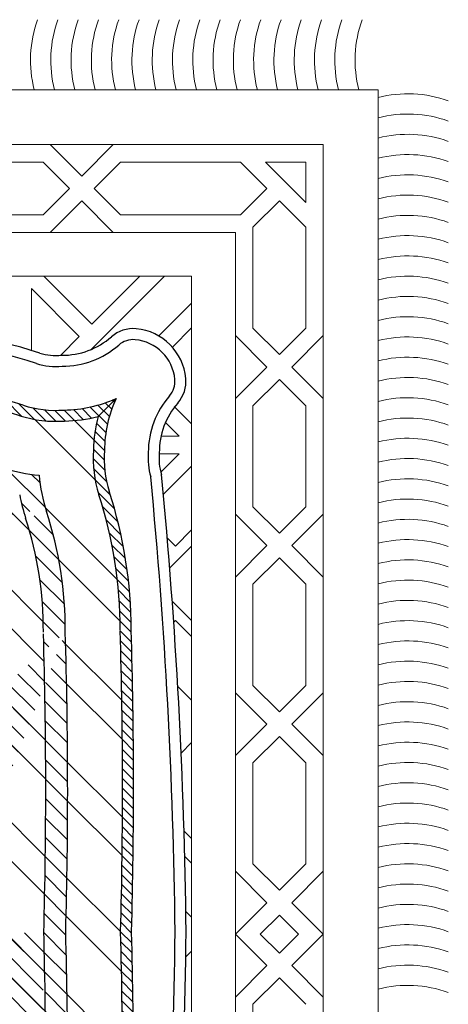
# Model space of a CAD drawing. Units: inches. Extents: x 3592 to 4861, y 1650 to 2243.
# Tile 8 of 30: x 4207 to 4219, y 1932 to 1959. Entities that reach past the tile are written whole.
import ezdxf

# ---------------------------------------------------------------- set-up
doc = ezdxf.new("R2010")
doc.units = ezdxf.units.IN
doc.layers.add('A-FURN', color=9, linetype='Continuous', lineweight=13)
doc.layers.add('RA-AP-01$0$INT', color=35, linetype='Continuous', lineweight=5)
for name, color, linetype in [('RA-AP-01$0$FURN', 3, 'Continuous'), ('RA-AP-01$0$WOOD', 64, 'Continuous'), ('RA-AP-02$0$FLPT', 30, 'Continuous')]:
    doc.layers.add(name, color=color, linetype=linetype)

# ---------------------------------------------------------------- blocks, each defined once
blk = doc.blocks.new('A$C67D63ADA')
at = {"layer": 'RA-AP-01$0$INT'}
for p, q in [((4.360068427138701, -6.272102561815665), (4.331382135641587, -6.243416270309323)), ((4.388754718643982, -6.243416270319609), (4.360068427138701, -6.272102561815665)), ((4.494210562764795, -6.243416270339973), (4.52289685426085, -6.272102561845255)), ((4.551583145766129, -6.243416270324172), (4.522896854260848, -6.272102561820228)), ((4.657038989890581, -6.243416270339336), (4.685725281386635, -6.272102561844619)), ((4.714411572875414, -6.243416270339336), (4.685725281379359, -6.272102561844619)), ((4.819867416996229, -6.243416270324516), (4.848553708501509, -6.272102561820572)), ((4.848553708501509, -6.272102561820572), (4.877239999998625, -6.243416270314227)), ((4.905926291512142, -6.272102561820572), (4.877240000015027, -6.243416270314227)), ((4.934612583017423, -6.243416270324516), (4.905926291512142, -6.272102561820572)), ((4.173240000009217, -6.296102561814969), (4.209926291520478, -6.259416270315509)), ((4.209926291520478, -6.259416270315509), (4.173240000009216, -6.259416270315509)), ((4.173240000009217, -6.296102561814969), (4.173240000009216, -6.259416270315509)), ((4.232553708503005, -6.259416270315509), (4.208553708513718, -6.283416270312518)), ((4.324754718648297, -6.259416270315509), (4.232553708503005, -6.259416270315509)), ((4.348754718637899, -6.283416270312828), (4.324754718648297, -6.259416270315509)), ((4.395382135631553, -6.2594162703285), (4.371382135635868, -6.283416270316472)), ((4.48758314576926, -6.259416270343913), (4.395382135631553, -6.2594162703285)), ((4.48758314576926, -6.259416270343913), (4.511583145760048, -6.283416270342422)), ((4.558210562765816, -6.259416270320948), (4.534210562758016, -6.283416270321034)), ((4.650411572888129, -6.259416270336362), (4.558210562765816, -6.259416270320948)), ((4.650411572888129, -6.259416270336362), (4.674411572885833, -6.283416270341786)), ((4.721038989873787, -6.25941627034044), (4.697038989880161, -6.283416270341786)), ((4.721038989873787, -6.25941627034044), (4.813239999999876, -6.259416270325027)), ((4.813240000000789, -6.259416270325538), (4.837240000004343, -6.283416270321379)), ((4.859867417002312, -6.283416270317736), (4.877240000001861, -6.2660436873126)), ((4.89461258301134, -6.283416270317736), (4.877240000011791, -6.2660436873126)), ((4.941240000012863, -6.259416270325538), (4.917240000009309, -6.283416270321379)), ((4.232553708510282, -6.307416270316805), (4.208553708513718, -6.283416270312518)), ((4.348754718637899, -6.283416270312828), (4.324754718627222, -6.307416270315791)), ((4.395382135640173, -6.307416270328503), (4.371382135635868, -6.283416270316472)), ((4.487583145750843, -6.307416270343915), (4.511583145760048, -6.283416270342422)), ((4.558210562750208, -6.307416270320947), (4.534210562758016, -6.283416270321034)), ((4.650411572883545, -6.307416270336361), (4.674411572885833, -6.283416270341786)), ((4.721038989886534, -6.307416270340442), (4.697038989880161, -6.283416270341786)), ((4.813240000007903, -6.30741627032554), (4.837240000004343, -6.283416270321379)), ((4.859867417002312, -6.283416270317736), (4.877240000006826, -6.300788853316665)), ((4.89461258301134, -6.283416270317736), (4.877240000006826, -6.300788853316665)), ((4.941240000005749, -6.30741627032554), (4.917240000009309, -6.283416270321379)), ((4.173240000009217, -6.318729978809296), (4.19724000000369, -6.294729978822545)), ((4.221240000009218, -6.318729978820355), (4.19724000000369, -6.294729978822545)), ((4.360068427135066, -6.294729978813635), (4.331382135628725, -6.323416270310751)), ((4.388754718631812, -6.323416270319609), (4.360068427135066, -6.294729978813635)), ((4.49421056275124, -6.323416270339973), (4.522896854257212, -6.294729978843224)), ((4.551583145753959, -6.323416270324171), (4.522896854257213, -6.294729978818199)), ((4.657038989877026, -6.323416270339336), (4.685725281382997, -6.294729978842587)), ((4.714411572888969, -6.323416270339336), (4.685725281382997, -6.294729978842587)), ((4.819867417008399, -6.323416270324515), (4.848553708505145, -6.294729978818542)), ((4.848553708505147, -6.29472997881854), (4.877240000011487, -6.323416270315655)), ((4.905926291508504, -6.29472997881854), (4.877240000002164, -6.323416270315655)), ((4.934612583005253, -6.323416270324515), (4.905926291508508, -6.294729978818542)), ((4.232553708510282, -6.307416270316805), (4.324754718627222, -6.307416270315791)), ((4.487583145750843, -6.307416270343915), (4.395382135640173, -6.307416270328503)), ((4.650411572883545, -6.307416270336361), (4.558210562750208, -6.307416270320947)), ((4.721038989886534, -6.307416270340442), (4.813240000007903, -6.307416270325028)), ((5.033441010127117, -6.307416270340442), (4.941240000005749, -6.307416270325028)), ((4.173240000009216, -6.428102561824165), (4.173240000009217, -6.318729978809296)), ((4.221240000009218, -6.428102561821944), (4.221240000009218, -6.318729978820355)), ((4.237240000008252, -6.353816270320467), (4.237240000008252, -6.933016270323148)), ((4.237240000008253, -6.353816270322416), (4.237240000008253, -6.933016270318608)), ((4.277240000006364, -6.923416270324413), (4.277240000021174, -6.363416270332882)), ((4.877240000006826, -6.363416270330311), (4.277240000021174, -6.363416270332882)), ((4.331724248037607, -6.393331975860947), (4.301808542509442, -6.363416270332777)), ((4.324435959507737, -6.36341627033268), (4.341921384137314, -6.380901694962252)), ((4.411867417009952, -6.363416270332308), (4.396098836564792, -6.379184850777471)), ((4.45049483400792, -6.363416270332143), (4.476136761714619, -6.389058198038839)), ((4.508671457515881, -6.363416270331893), (4.45049483400792, -6.363416270332143)), ((4.508671457515881, -6.363416270331891), (4.523298874513887, -6.378043687329895)), ((4.591181125507156, -6.363416270331923), (4.523298874513629, -6.363416270331545)), ((4.543172726528447, -6.383290122346805), (4.523298874513629, -6.363416270331545)), ((4.573619639006339, -6.380977756832742), (4.591181125507156, -6.363416270331923)), ((4.605808542505038, -6.363416270331884), (4.591181125507032, -6.378043687329889)), ((4.591181125507033, -6.378043687329889), (4.605808542505001, -6.363416270331923)), ((4.605808542505038, -6.363416270331886), (4.663985166013, -6.363416270332124)), ((4.663985166013, -6.363416270332124), (4.65146504581717, -6.375936390527956)), ((4.702612583010965, -6.36341627033228), (4.790044040513182, -6.363416270332642)), ((4.702612583010966, -6.363416270332284), (4.712072573448597, -6.372876260769913)), ((4.790044040513182, -6.363416270332642), (4.783212045294504, -6.370248265551321)), ((4.806473209246069, -6.369614518597721), (4.812671457513201, -6.363416270330588)), ((4.856598418256279, -6.368626394577383), (4.861808542503284, -6.363416270330378)), ((4.877240000006826, -6.363416270330311), (5.477239999992479, -6.363416270332882)), ((4.897949975524354, -6.368694788344366), (4.892671457510368, -6.363416270330378)), ((4.423181125509032, -6.374729978831202), (4.410714462749727, -6.387196641590509)), ((4.423181125509103, -6.391217225305457), (4.423181125509032, -6.374729978831202)), ((4.439181125509032, -6.374729978831223), (4.455879744643261, -6.39142859796545)), ((4.43918112550911, -6.392862294450365), (4.439181125509032, -6.374729978831223)), ((4.51581063184268, -6.385531930001103), (4.523298874513885, -6.378043687329895)), ((4.592759677987533, -6.379622239810387), (4.591181125507033, -6.378043687329889)), ((4.344016470827723, -6.454761283640936), (4.277240000020523, -6.387984812833736)), ((4.277240000019926, -6.410612229819946), (4.320955728769878, -6.454327958571846)), ((4.173240000009216, -6.428102561824165), (4.197240000007798, -6.452102561823052)), ((4.221240000009218, -6.428102561821944), (4.197240000007798, -6.452102561823052)), ((4.157240000008254, -6.434729978821112), (4.185926291507684, -6.463416270320908)), ((4.237240000008253, -6.434729978820932), (4.20855370850791, -6.46341627032091)), ((4.277240000017616, -6.498043687322161), (4.320955728769878, -6.454327958571846)), ((4.157240000008254, -6.492102561820703), (4.185926291507684, -6.463416270320908)), ((4.237240000008253, -6.492102561820884), (4.20855370850791, -6.46341627032091)), ((4.28855370851626, -6.509357395821494), (4.332269437268611, -6.465641667071082)), ((4.332269437268613, -6.465641667071083), (4.349438136078297, -6.482810365881532)), ((4.173240000008253, -6.498729978818613), (4.197240000007798, -6.474729978818764)), ((4.221240000008254, -6.498729978818907), (4.197240000007798, -6.474729978818764)), ((4.173240000008255, -6.608102561821608), (4.173240000008253, -6.498729978818613)), ((4.221240000008257, -6.608102561821311), (4.221240000008254, -6.498729978818907)), ((4.344903410716357, -6.509357395822983), (4.28855370851626, -6.509357395821494))]:
    blk.add_line(p, q, dxfattribs=at)
for points in [[(5.647240000006826, -6.243416270325369), (5.647240000006826, -7.09341627032537), (4.107240000006826, -7.093416270325372), (4.107240000006826, -6.19341627032537), (4.877240000006826, -6.19341627032537)], [(4.877240000006826, -6.19341627032537), (5.647240000006826, -6.19341627032537), (5.647240000006826, -7.09341627032537), (4.877240000006826, -7.09341627032537)], [(5.597240000006826, -6.243416270325369), (5.597240000006826, -7.04341627032537), (4.157240000006826, -7.043416270325372), (4.157240000006826, -6.243416270325369)], [(4.877240000006826, -6.243416270325369), (4.157240000006826, -6.243416270325369)], [(4.877240000006826, -6.243416270325369), (5.597240000006826, -6.243416270325369)], [(4.877240000006826, -6.32341627032537), (4.237240000006825, -6.32341627032537), (4.237240000006825, -6.963416270325371), (4.877240000006826, -6.963416270325371)], [(4.877240000006826, -6.32341627032537), (5.517240000006826, -6.32341627032537), (5.517240000006826, -6.963416270325371), (4.877240000006826, -6.963416270325371)]]:
    blk.add_lwpolyline(points, dxfattribs=at)
for centre, start, end in [((4.220001958960506, -6.166456270323309), 160.2038431294313, 194.3025426369059), ((4.238481958959505, -6.166456270325492), 160.2038431294313, 194.302542635723), ((4.256961958958505, -6.166456270325492), 160.2038431294313, 194.302542635723), ((4.275441958962233, -6.166456270324219), 160.2038431294313, 194.3025426364132), ((4.293921958961232, -6.166456270326402), 160.2038431294313, 194.3025426352303), ((4.312401958960231, -6.166456270326402), 160.2038431294313, 194.3025426352303), ((4.33088195896396, -6.166456270325128), 160.2038431294313, 194.3025426359204), ((4.349361958962959, -6.166456270326038), 160.2038431294313, 194.3025426354275), ((4.367841958959411, -6.166456270326038), 160.2038431294313, 194.3025426354275), ((4.386321958963322, -6.166456270324765), 160.2038431294313, 194.3025426361172), ((4.404801958962321, -6.166456270326947), 160.2038431294313, 194.3025426349348), ((4.42328195896132, -6.166456270326947), 160.2038431294313, 194.3025426349348), ((4.441761958965049, -6.166456270325674), 160.2038431294313, 194.3025426356244), ((4.460241958964048, -6.166456270326584), 160.2038431294313, 194.3025426351316), ((4.4787219589605, -6.166456270326584), 160.2038431294313, 194.3025426351316), ((4.497201958964411, -6.16645627032531), 160.2038431294313, 194.3025426358216), ((4.515681958963228, -6.166456270323855), 160.2038431294313, 194.3025426366099), ((4.534161958959862, -6.16645627032622), 160.2038431294313, 194.3025426353289), ((4.552641958963591, -6.166456270326038), 160.2038431294313, 194.3025426354275), ((4.571121958962589, -6.166456270324765), 160.2038431294313, 194.3025426361172), ((4.589601958963954, -6.166456270323491), 160.2038431294313, 194.3025426368072), ((4.608081958962952, -6.166456270325674), 160.2038431294313, 194.3025426356244), ((4.626561958963465, -6.166456270323128), 160.2038431294313, 194.3025426370041), ((4.626561958964317, -6.166456270325492), 160.2038431294313, 194.302542635723), ((4.645041958962464, -6.16645627032531), 160.2038431294313, 194.3025426358216), ((4.663521958961464, -6.16645627032531), 160.2038431294313, 194.3025426358216), ((4.682001958965192, -6.166456270324037), 160.2038431294313, 194.3025426365113), ((4.700481958964191, -6.166456270324947), 160.2038431294313, 194.3025426360186), ((4.718961958960644, -6.166456270324947), 160.2038431294313, 194.3025426360186), ((4.737441958964554, -6.166456270323673), 160.2038431294313, 194.3025426367086), ((4.755921958963371, -6.166456270322218), 160.2038431294313, 194.3025426374968), ((4.774401958960006, -6.166456270324583), 160.2038431294313, 194.3025426362158), ((4.792881958963734, -6.166456270324401), 160.2038431294313, 194.3025426363144), ((4.811361958962733, -6.166456270323128), 160.2038431294313, 194.3025426370041), ((4.829841958964097, -6.166456270321854), 160.2038431294313, 194.3025426376941), ((4.848321958963096, -6.166456270324037), 160.2038431294313, 194.3025426365113), ((4.86680195896446, -6.166456270323855), 160.2038431294313, 194.3025426366099), ((4.885281958960913, -6.16645627032149), 160.2038431294313, 194.3025426378914), ((4.903761958964823, -6.166456270321309), 160.2038431294313, 194.3025426379896), ((4.92224195896364, -6.166456270323673), 160.2038431294313, 194.3025426367086), ((4.940721958962639, -6.1664562703224), 160.2038431294313, 194.3025426373987), ((4.959201958964003, -6.166456270320945), 160.2038431294313, 194.3025426381869), ((4.977681958963002, -6.166456270320945), 160.2038431294313, 194.3025426381869), ((4.996161958962002, -6.166456270323128), 160.2038431294313, 194.3025426370041), ((5.014641958961001, -6.166456270323128), 160.2038431294313, 194.3025426370041), ((5.033121958964729, -6.166456270321854), 160.2038431294313, 194.3025426376941), ((4.080280000008716, -6.105294311367939), 250.2038431288995, 284.3025426347654), ((4.080280000011353, -6.123774311370394), 250.2038431288995, 284.3025426333367), ((4.080280000008989, -6.142254311367028), 250.2038431288995, 284.3025426346176), ((4.080280000006625, -6.160734311363481), 250.2038431288995, 284.3025426358987), ((4.080280000009262, -6.179214311365936), 250.2038431288995, 284.3025426344699), ((4.080280000006897, -6.19769431136257), 250.2038431288995, 284.302542635751), ((4.080280000004532, -6.216174311359023), 250.2038431288995, 284.3025426370325), ((4.080280000007079, -6.234654311360387), 250.2038431288995, 284.3025426356524), ((4.08028000000726, -6.253134311360659), 250.2038431288995, 284.3025426355542), ((4.08028000000726, -6.271614311362022), 250.2038431288995, 284.3025426355542), ((4.080280000005078, -6.290094311364478), 250.2038431288995, 284.3025426367365), ((4.080280000007534, -6.30857431136475), 250.2038431288995, 284.302542635406), ((4.080280000007625, -6.327054311362476), 250.2038431288995, 284.3025426353568), ((4.080280000005441, -6.345534311362567), 250.2038431288995, 284.3025426365397), ((4.080280000005533, -6.364014311362839), 250.2038431288995, 284.3025426364901), ((4.080280000005624, -6.382494311361838), 250.2038431288995, 284.302542636441), ((4.08028000000817, -6.400974311363202), 250.2038431288995, 284.3025426350613)]:
    blk.add_arc(centre, 0.1091312342836184, start, end, dxfattribs=at)
blk = doc.blocks.new('A$C09A87C41')
at = {"layer": 'RA-AP-01$0$WOOD'}
h = blk.add_hatch(dxfattribs=at)
h.set_pattern_fill('ANSI31', color=256, scale=0.05, style=0)
h.set_pattern_definition([(45, (0.7182879904584168, -11.54818755465011), (0.0044194173824159, -0.0044194173824159), [])])
edge = h.paths.add_edge_path()
edge.add_ellipse((5.006516613079209, -11.27459283286495), major_axis=(3.435359877543153, 3.435359877543153), ratio=0.9999999999999982, start_angle=403.3022422558093, end_angle=406.5486575131389, ccw=False)
edge.add_ellipse((5.150455045735207, -6.828790194879051), major_axis=(-0.2901946312779826, 0.2901946312779826), ratio=0.9999999999999875, start_angle=297.2093186994243, end_angle=314.9999999999731, ccw=False)
edge.add_ellipse((5.307117976013378, -6.343033378039902), major_axis=(-0.0707106781186454, 0.0707106781186455), ratio=0.9999999999999651, start_angle=116.7779839927149, end_angle=139.0873288843009)
edge.add_ellipse((5.312718414970339, -6.324818905441738), major_axis=(0.0834173982641243, 0.0834173982641243), ratio=0.9999999999999847, start_angle=225.741775187377, end_angle=249.5633269497028)
edge.add_line((5.361758401537698, -6.432112914518591), (5.345299417747169, -6.448571898309089))
edge.add_ellipse((5.312718414970311, -6.32481890544173), major_axis=(-0.0904884660759946, 0.0904884660759945), ratio=0.9999999999999644, start_angle=135.8720682536374, end_angle=149.7498089726665, ccw=False)
edge.add_ellipse((5.307117976013483, -6.343033378039922), major_axis=(-0.0777817459304867, 0.0777817459304867), ratio=0.9999999999999941, start_angle=117.45144083316339, end_angle=138.9346900893823, ccw=False)
edge.add_ellipse((5.150455045735208, -6.82879019487905), major_axis=(0.2831235634661059, 0.2831235634661059), ratio=0.9999999999999859, start_angle=27.03507540014952, end_angle=44.9867285887044)
edge.add_ellipse((5.006516315412802, -11.27459997798134), major_axis=(-3.428298916554014, 3.428298916554014), ratio=0.9999999999999971, start_angle=-46.70235550375367, end_angle=-43.44815559494434)
edge.add_ellipse((4.743915471599394, -11.2745999779814), major_axis=(3.428298916553931, 3.42829891655393), ratio=0.9999999999999994, start_angle=43.44815559494427, end_angle=46.70235550375375)
edge.add_ellipse((4.599976741276995, -6.828790194879051), major_axis=(0.2831235634661173, 0.2831235634661172), ratio=0.9999999999999861, start_angle=45.01327141129749, end_angle=62.96492459984043)
edge.add_ellipse((4.443313810998718, -6.343033378039922), major_axis=(0.0777817459304893, 0.0777817459304893), ratio=0.9999999999999873, start_angle=221.0653099106178, end_angle=242.54855916687399, ccw=False)
edge.add_ellipse((4.437713372041892, -6.32481890544173), major_axis=(0.0904884660759951, 0.0904884660759951), ratio=0.9999999999999603, start_angle=210.2501910273332, end_angle=224.1279317463614, ccw=False)
edge.add_line((4.405132369265034, -6.448571898309089), (4.388673385474508, -6.432112914518594))
edge.add_ellipse((4.43771337204186, -6.324818905441737), major_axis=(0.0834173982641232, 0.0834173982641232), ratio=0.9999999999999797, start_angle=200.4366730503009, end_angle=224.2582248126243)
edge.add_ellipse((4.443313810998827, -6.343033378039902), major_axis=(-0.0707106781186382, 0.0707106781186382), ratio=0.9999999999999952, start_angle=130.9126711156974, end_angle=153.2220160072772)
edge.add_ellipse((4.599976741276995, -6.828790194879051), major_axis=(-0.2901946312779718, 0.2901946312779718), ratio=0.9999999999999895, start_angle=315.0000000000233, end_angle=332.7906813005773, ccw=False)
edge.add_ellipse((4.743915173933024, -11.27459283286497), major_axis=(-3.435359877543123, 3.435359877543123), ratio=0.9999999999999991, start_angle=313.451342486861, end_angle=316.69775774419077, ccw=False)
edge = h.paths.add_edge_path()
edge.add_ellipse((4.299593848995801, -6.48675334004306), major_axis=(-0.0707106781186556, 0.0707106781186556), ratio=0.9999999999999859, start_angle=206.7779839906583, end_angle=229.0873288838364)
edge.add_ellipse((4.281379376397651, -6.481152901086075), major_axis=(-0.0834173982641623, 0.0834173982641623), ratio=0.9999999999999754, start_angle=225.7417751869729, end_angle=249.5633269497573)
edge.add_line((4.388673385474506, -6.432112914518592), (4.405132369265034, -6.448571898309089))
edge.add_ellipse((4.281379376397657, -6.481152901086004), major_axis=(-0.0904884660760182, 0.0904884660760182), ratio=0.9999999999999957, start_angle=225.8720682533453, end_angle=239.7498089726896, ccw=False)
edge.add_ellipse((4.299593848995796, -6.486753340043026), major_axis=(0.0777817459305317, 0.0777817459305317), ratio=0.9999999999999891, start_angle=297.4514408381613, end_angle=318.9346900891407, ccw=False)
edge.add_ellipse((4.785350665835052, -6.643416270320893), major_axis=(0.2831235634661102, 0.2831235634661102), ratio=0.9999999999999978, start_angle=117.0350753988375, end_angle=152.9649246009711)
edge.add_ellipse((4.299593848995777, -6.800079200598784), major_axis=(-0.0777817459305426, 0.0777817459305426), ratio=0.9999999999999973, start_angle=221.0653099111909, end_angle=242.5485591625442, ccw=False)
edge.add_ellipse((4.281379376397679, -6.805679639555494), major_axis=(-0.0904884660760244, 0.0904884660760244), ratio=0.9999999999999076, start_angle=210.2501910270576, end_angle=224.1279317467988, ccw=False)
edge.add_line((4.405132369264926, -6.838260642332959), (4.388673385474263, -6.854719626123697))
edge.add_ellipse((4.281379376397679, -6.80567963955562), major_axis=(0.0834173982641642, 0.0834173982641642), ratio=0.9999999999999609, start_angle=290.4366730499258, end_angle=314.2582248131156)
edge.add_ellipse((4.299593848995804, -6.800079200598786), major_axis=(-0.0707106781186612, 0.0707106781186612), ratio=0.999999999999977, start_angle=220.9126711163551, end_angle=243.222016008517)
edge.add_ellipse((4.785350665835053, -6.643416270320894), major_axis=(0.2901946312779783, 0.2901946312779783), ratio=0.9999999999999984, start_angle=117.2093186999746, end_angle=152.7906813002342, ccw=False)
edge = h.paths.add_edge_path()
edge.add_ellipse((4.743915471599392, -2.012232562660299), major_axis=(3.428298916553894, 3.428298916553894), ratio=0.9999999999999992, start_angle=223.2976444962459, end_angle=226.5518444050561)
edge.add_ellipse((5.006516315412771, -2.012232562660296), major_axis=(3.428298916553752, 3.428298916553752), ratio=0.9999999999999971, start_angle=223.448155594945, end_angle=226.7023555037531)
edge.add_ellipse((5.150455045735209, -6.458042345762599), major_axis=(0.283123563466111, 0.283123563466111), ratio=0.999999999999996, start_angle=225.0132714112834, end_angle=242.9649246011241)
edge.add_ellipse((5.30711797601273, -6.94379916260194), major_axis=(0.0777817459305174, 0.0777817459305174), ratio=0.9999999999999873, start_angle=401.06530991071423, end_angle=422.548559161793, ccw=False)
edge.add_ellipse((5.312718414969516, -6.962013635200094), major_axis=(0.0904884660760023, 0.0904884660760023), ratio=0.9999999999999566, start_angle=390.2501910269164, end_angle=404.12793174642553, ccw=False)
edge.add_line((5.345299417747278, -6.838260642332959), (5.361758401537942, -6.854719626123698))
edge.add_ellipse((5.312718414969516, -6.962013635200098), major_axis=(0.0834173982641439, 0.0834173982641439), ratio=0.9999999999999785, start_angle=20.43667304973462, end_angle=44.25822481258737)
edge.add_ellipse((5.307117976012772, -6.943799162601948), major_axis=(-0.0707106781186618, 0.0707106781186618), ratio=0.999999999999977, start_angle=-49.08732888421749, end_angle=-26.77798399064677)
edge.add_ellipse((5.150455045735209, -6.458042345762597), major_axis=(0.2901946312779783, 0.2901946312779783), ratio=0.9999999999999957, start_angle=225.0000000000273, end_angle=242.7906812999824, ccw=False)
edge.add_ellipse((5.006516613079198, -2.012239707776725), major_axis=(3.43535987754352, 3.43535987754352), ratio=0.999999999999996, start_angle=223.4513424868609, end_angle=226.697757744191, ccw=False)
edge.add_ellipse((4.743915173933023, -2.012239707776712), major_axis=(3.435359877543229, 3.435359877543229), ratio=0.9999999999999998, start_angle=223.3022422558095, end_angle=226.5486575131387, ccw=False)
edge.add_ellipse((4.599976741276995, -6.458042345762597), major_axis=(0.2901946312779746, 0.2901946312779748), ratio=0.9999999999999964, start_angle=207.2093187000184, end_angle=224.9999999999795, ccw=False)
edge.add_ellipse((4.443313810999427, -6.943799162601947), major_axis=(-0.070710678118668, 0.070710678118668), ratio=0.9999999999999838, start_angle=-63.22201600935903, end_angle=-40.9126711157662)
edge.add_ellipse((4.437713372042683, -6.962013635200099), major_axis=(0.0834173982641484, 0.0834173982641484), ratio=0.9999999999999729, start_angle=45.74177518742643, end_angle=69.56332695026246)
edge.add_line((4.388673385474263, -6.854719626123697), (4.405132369264926, -6.838260642332958))
edge.add_ellipse((4.437713372042681, -6.962013635200094), major_axis=(0.0904884660760224, 0.0904884660760225), ratio=0.9999999999999282, start_angle=405.87206825357924, end_angle=419.7498089730807, ccw=False)
edge.add_ellipse((4.443313810999475, -6.94379916260194), major_axis=(-0.0777817459305165, 0.0777817459305165), ratio=0.9999999999999927, start_angle=297.4514408382556, end_angle=318.93469008929503, ccw=False)
edge.add_ellipse((4.599976741276995, -6.458042345762597), major_axis=(0.2831235634661077, 0.2831235634661077), ratio=0.9999999999999937, start_angle=207.0350753988627, end_angle=224.9867285886981)
edge = h.paths.add_edge_path()
edge.add_ellipse((5.450837938016399, -6.800079200598789), major_axis=(-0.0707106781186565, 0.0707106781186565), ratio=0.9999999999999875, start_angle=26.77798399147072, end_angle=49.08732888364846)
edge.add_ellipse((5.469052410614524, -6.80567963955562), major_axis=(0.0834173982641601, 0.0834173982641601), ratio=0.9999999999999984, start_angle=135.7417751868887, end_angle=159.563326950074)
edge.add_line((5.36175840153794, -6.854719626123697), (5.345299417747278, -6.838260642332959))
edge.add_ellipse((5.469052410614523, -6.805679639555488), major_axis=(0.0904884660760307, 0.0904884660760307), ratio=0.9999999999999984, start_angle=135.8720682531977, end_angle=149.7498089729454, ccw=False)
edge.add_ellipse((5.450837938016426, -6.800079200598787), major_axis=(0.0777817459305426, 0.0777817459305427), ratio=0.9999999999999968, start_angle=117.4514408374904, end_angle=138.9346900888003, ccw=False)
edge.add_ellipse((4.965081121177151, -6.643416270320895), major_axis=(-0.2831235634661119, 0.2831235634661119), ratio=0.9999999999999992, start_angle=207.0350753990193, end_angle=242.9649246011595)
edge.add_ellipse((5.450837938016407, -6.486753340043026), major_axis=(0.0777817459305285, 0.0777817459305285), ratio=0.9999999999999747, start_angle=131.0653099108597, end_angle=152.5485591618505, ccw=False)
edge.add_ellipse((5.469052410614547, -6.481152901086004), major_axis=(0.09048846607603, 0.09048846607603), ratio=0.9999999999999619, start_angle=120.25019102731059, end_angle=134.1279317466551, ccw=False)
edge.add_line((5.345299417747169, -6.448571898309089), (5.361758401537697, -6.432112914518592))
edge.add_ellipse((5.469052410614551, -6.481152901086075), major_axis=(-0.0834173982641603, 0.0834173982641603), ratio=0.9999999999999998, start_angle=20.43667305024269, end_angle=44.25822481302925)
edge.add_ellipse((5.450837938016403, -6.486753340043062), major_axis=(-0.0707106781186603, 0.0707106781186603), ratio=0.9999999999999737, start_angle=40.91267111616517, end_angle=63.22201600943157)
edge.add_ellipse((4.965081121177149, -6.643416270320895), major_axis=(0.2901946312779771, 0.2901946312779771), ratio=0.9999999999999992, start_angle=297.2093186997686, end_angle=332.7906813000034, ccw=False)
h = blk.add_hatch(dxfattribs=at)
h.set_pattern_fill('ANSI32', color=256, scale=0.2, style=0)
h.set_pattern_definition([(45, (0.7182879904584168, -11.54818755465011), (0.0530330085889911, -0.0530330085889911), []), (45, (0.7182879904584168, -11.51283221565011), (0.0530330085889911, -0.0530330085889911), [])])
edge = h.paths.add_edge_path()
edge.add_ellipse((5.15045504573521, -6.82879019487905), major_axis=(-0.2831235634661157, 0.2831235634661156), ratio=0.9999999999999889, start_angle=297.21454354460053, end_angle=314.98672858870884, ccw=False)
edge.add_ellipse((5.307117976013485, -6.343033378039922), major_axis=(-0.0777817459304881, 0.0777817459304881), ratio=0.9999999999999928, start_angle=116.7981781115797, end_angle=138.9346900893818)
edge.add_ellipse((5.312718414970311, -6.32481890544173), major_axis=(-0.0904884660759946, 0.0904884660759946), ratio=0.9999999999999658, start_angle=135.8720682536378, end_angle=149.7498089726664)
edge.add_ellipse((5.469052410614547, -6.481152901086004), major_axis=(0.0904884660760303, 0.0904884660760302), ratio=0.9999999999999603, start_angle=120.2501910273106, end_angle=134.1279317466551)
edge.add_ellipse((5.450837938016407, -6.486753340043026), major_axis=(-0.0777817459305327, 0.0777817459305327), ratio=0.9999999999999915, start_angle=41.06530991085969, end_angle=63.20182189333976)
edge.add_ellipse((4.965081121177151, -6.643416270320894), major_axis=(-0.2831235634661133, 0.2831235634661133), ratio=0.9999999999999984, start_angle=207.214543545815, end_angle=242.7854564539869, ccw=False)
edge.add_ellipse((5.450837938016426, -6.800079200598786), major_axis=(0.0777817459305424, 0.0777817459305424), ratio=0.9999999999999962, start_angle=116.7981781073729, end_angle=138.9346900888086)
edge.add_ellipse((5.469052410614524, -6.805679639555493), major_axis=(0.0904884660760289, 0.0904884660760289), ratio=0.9999999999999841, start_angle=135.872068253202, end_angle=149.7498089729424)
edge.add_ellipse((5.312718414969522, -6.962013635200094), major_axis=(-0.0904884660760224, 0.0904884660760225), ratio=0.9999999999999282, start_angle=-59.7498089730807, end_angle=-45.87206825357926)
edge.add_ellipse((5.307117976012728, -6.94379916260194), major_axis=(0.0777817459305181, 0.0777817459305181), ratio=0.9999999999999861, start_angle=41.06530991070497, end_angle=63.20182189334603)
edge.add_ellipse((5.150455045735208, -6.458042345762599), major_axis=(0.2831235634661146, 0.2831235634661146), ratio=0.9999999999999907, start_angle=225.013271411291, end_angle=242.7854564539341, ccw=False)
edge.add_ellipse((5.006516315412806, -2.012232562660296), major_axis=(3.428298916554143, 3.428298916554143), ratio=0.9999999999999941, start_angle=223.4481555949448, end_angle=226.7023555037533, ccw=False)
edge.add_ellipse((4.743915471599424, -2.012232562660299), major_axis=(3.428298916554168, 3.428298916554171), ratio=0.9999999999999991, start_angle=223.2976444962462, end_angle=226.551844405056, ccw=False)
edge.add_ellipse((4.599976741276996, -6.458042345762597), major_axis=(0.2831235634661098, 0.2831235634661098), ratio=0.9999999999999973, start_angle=207.2145435460398, end_angle=224.9867285887048, ccw=False)
edge.add_ellipse((4.443313810999473, -6.94379916260194), major_axis=(-0.0777817459305183, 0.0777817459305183), ratio=0.9999999999999823, start_angle=-63.2018218932521, end_angle=-41.06530991071377)
edge.add_ellipse((4.437713372042686, -6.962013635200094), major_axis=(-0.0904884660760028, 0.0904884660760028), ratio=0.9999999999999504, start_angle=-44.12793174642511, end_angle=-30.25019102691602)
edge.add_ellipse((4.281379376397679, -6.80567963955549), major_axis=(-0.0904884660760215, 0.0904884660760215), ratio=0.9999999999999245, start_angle=210.2501910270558, end_angle=224.1279317467963)
edge.add_ellipse((4.299593848995777, -6.800079200598786), major_axis=(0.077781745930539, 0.077781745930539), ratio=0.999999999999963, start_angle=311.0653099111909, end_angle=333.2018218926339)
edge.add_ellipse((4.785350665835052, -6.643416270320894), major_axis=(0.2831235634661089, 0.2831235634661091), ratio=0.9999999999999989, start_angle=117.21454354600829, end_angle=152.7854564541833, ccw=False)
edge.add_ellipse((4.299593848995796, -6.486753340043026), major_axis=(0.077781745930533, 0.077781745930533), ratio=0.9999999999999792, start_angle=296.7981781066777, end_angle=318.9346900891398)
edge.add_ellipse((4.281379376397657, -6.481152901086003), major_axis=(-0.0904884660760217, 0.0904884660760217), ratio=0.9999999999999742, start_angle=225.872068253344, end_angle=239.7498089726891)
edge.add_ellipse((4.437713372041892, -6.32481890544173), major_axis=(0.090488466075997, 0.090488466075997), ratio=0.9999999999999756, start_angle=210.2501910273331, end_angle=224.1279317463622)
edge.add_ellipse((4.44331381099872, -6.343033378039923), major_axis=(0.0777817459304873, 0.0777817459304872), ratio=0.9999999999999861, start_angle=221.0653099106177, end_angle=243.2018218883976)
edge.add_ellipse((4.599976741276995, -6.828790194879051), major_axis=(-0.2831235634661067, 0.2831235634661067), ratio=0.9999999999999895, start_angle=315.01327141129775, end_angle=332.78545645540567, ccw=False)
edge.add_ellipse((4.743915471599392, -11.2745999779814), major_axis=(-3.428298916553902, 3.428298916553902), ratio=0.9999999999999984, start_angle=313.4481555949443, end_angle=316.7023555037538, ccw=False)
edge.add_ellipse((5.006516315412786, -11.27459997798134), major_axis=(-3.428298916554052, 3.428298916554052), ratio=1, start_angle=313.29764449624645, end_angle=316.5518444050555, ccw=False)
edge = h.paths.add_edge_path(flags=16)
edge.add_ellipse((4.745320840887742, -11.27459782170807), major_axis=(3.392940520945516, 3.392940520945516), ratio=1, start_angle=43.44876692339471, end_angle=46.71249975461917)
edge.add_ellipse((4.599976741276995, -6.828790194878992), major_axis=(-0.2477682244067734, 0.2477682244067734), ratio=0.9999999999999911, start_angle=-45.31868720933983, end_angle=-27.00912183057358)
edge.add_ellipse((4.443313810998828, -6.343033378039872), major_axis=(0.1131370849898469, 0.1131370849898469), ratio=0.9999999999999724, start_angle=230.5682590208478, end_angle=242.6218359751805, ccw=False)
edge.add_ellipse((4.299593848995757, -6.486753340043112), major_axis=(-0.1131370849898624, 0.1131370849898624), ratio=0.9999999999999953, start_angle=207.3781640250758, end_angle=219.4317409792351, ccw=False)
edge.add_ellipse((4.78535066583505, -6.643416270320884), major_axis=(0.2477682244067863, 0.2477682244067863), ratio=0.9999999999999974, start_angle=117.0091218305267, end_angle=152.9908781690427)
edge.add_ellipse((4.299593848995773, -6.800079200598856), major_axis=(0.1131370849898833, 0.1131370849898833), ratio=0.9999999999999682, start_angle=320.56825902084296, end_angle=332.62183597593753, ccw=False)
edge.add_ellipse((4.443313810999473, -6.943799162601939), major_axis=(0.1131370849898351, 0.1131370849898351), ratio=0.9999999999999213, start_angle=387.3781640246361, end_angle=399.43174097937606, ccw=False)
edge.add_ellipse((4.599976741276996, -6.458042345762606), major_axis=(0.2477682244067743, 0.2477682244067742), ratio=0.99999999999999, start_angle=207.0091218307682, end_angle=225.3186872093523)
edge.add_ellipse((4.745320840887777, -2.012234718933553), major_axis=(-3.392940520945741, 3.392940520945741), ratio=0.9999999999999992, start_angle=133.2875002453813, end_angle=136.5512330766047)
edge.add_ellipse((5.005110946124445, -2.012234718933546), major_axis=(3.392940520945412, 3.392940520945411), ratio=0.9999999999999989, start_angle=223.4487669233947, end_angle=226.7124997546191)
edge.add_ellipse((5.150455045735207, -6.458042345762608), major_axis=(-0.2477682244067739, 0.2477682244067739), ratio=0.9999999999999966, start_angle=134.6813127906568, end_angle=152.9908781692236)
edge.add_ellipse((5.30711797601273, -6.943799162601939), major_axis=(-0.1131370849898406, 0.1131370849898406), ratio=0.9999999999999811, start_angle=320.568259020624, end_angle=332.62183597538194, ccw=False)
edge.add_ellipse((5.45083793801643, -6.800079200598855), major_axis=(0.113137084989895, 0.113137084989895), ratio=0.999999999999955, start_angle=117.3781640240419, end_angle=129.4317409791577, ccw=False)
edge.add_ellipse((4.965081121177152, -6.643416270320884), major_axis=(0.2477682244067847, 0.2477682244067847), ratio=0.9999999999999992, start_angle=297.0091218309669, end_angle=332.990878169475)
edge.add_ellipse((5.450837938016447, -6.486753340043118), major_axis=(-0.1131370849898789, 0.1131370849898789), ratio=0.9999999999999342, start_angle=50.56825902076281, end_angle=62.62183597491821, ccw=False)
edge.add_ellipse((5.30711797601337, -6.34303337803987), major_axis=(0.1131370849898374, 0.1131370849898374), ratio=0.9999999999999493, start_angle=207.3781640247929, end_angle=219.4317409791543, ccw=False)
edge.add_ellipse((5.150455045735204, -6.828790194878992), major_axis=(-0.2477682244067807, 0.2477682244067808), ratio=0.9999999999999934, start_angle=-62.99087816941401, end_angle=-44.68131279065508)
edge.add_ellipse((5.005110946124442, -11.27459782170805), major_axis=(3.392940520945543, 3.392940520945543), ratio=0.9999999999999974, start_angle=43.28750024538099, end_angle=46.55123307660507)
edge = h.paths.add_edge_path(flags=0)
edge.add_ellipse((4.745321446260899, -11.27461227828643), major_axis=(3.378818834290158, 3.378818834290157), ratio=0.9999999999999996, start_angle=43.44228925150885, end_angle=46.72161971502517)
edge.add_ellipse((4.599976741276998, -6.828790194878991), major_axis=(-0.2336260887830454, 0.2336260887830454), ratio=0.9999999999999974, start_angle=-45.30974264369766, end_angle=-26.99844483641433)
edge.add_ellipse((4.443313810998811, -6.343033378039858), major_axis=(0.1272792206135962, 0.1272792206135962), ratio=0.9999999999999403, start_angle=235.6264990356023, end_angle=242.6432427499436, ccw=False)
edge.add_ellipse((4.299593848995773, -6.486753340043007), major_axis=(0.1272792206136285, 0.1272792206136286), ratio=0.9999999999999204, start_angle=297.35675724967757, end_angle=304.3735009644582, ccw=False)
edge.add_ellipse((4.785350665835048, -6.643416270320905), major_axis=(0.2336260887830504, 0.2336260887830504), ratio=0.9999999999999921, start_angle=116.998444836676, end_angle=153.0015551636886)
edge.add_ellipse((4.299593848995741, -6.800079200598703), major_axis=(-0.1272792206136906, 0.1272792206136906), ratio=0.9999999999996289, start_angle=235.62649903554922, end_angle=242.64324274961962, ccw=False)
edge.add_ellipse((4.443313810999469, -6.943799162601998), major_axis=(-0.1272792206136219, 0.1272792206136219), ratio=0.9999999999999658, start_angle=297.3567572500489, end_angle=304.3735009646209, ccw=False)
edge.add_ellipse((4.599976741276995, -6.458042345762605), major_axis=(0.2336260887830445, 0.2336260887830445), ratio=0.9999999999999957, start_angle=206.9984448365414, end_angle=225.3097426436968)
edge.add_ellipse((4.745321446260921, -2.012220262355212), major_axis=(3.378818834290089, 3.378818834290088), ratio=0.9999999999999994, start_angle=223.2783802849744, end_angle=226.5577107484907)
edge.add_ellipse((5.005110340751275, -2.012220262355198), major_axis=(3.378818834290274, 3.378818834290274), ratio=0.9999999999999992, start_angle=223.4422892515091, end_angle=226.7216197150253)
edge.add_ellipse((5.150455045735206, -6.458042345762609), major_axis=(0.2336260887830463, 0.2336260887830463), ratio=0.9999999999999937, start_angle=224.6902573562994, end_angle=243.0015551634542)
edge.add_ellipse((5.30711797601273, -6.943799162602), major_axis=(-0.1272792206135949, 0.1272792206135949), ratio=0.9999999999997138, start_angle=325.62649903537766, end_angle=332.6432427499585, ccw=False)
edge.add_ellipse((5.450837938016461, -6.800079200598699), major_axis=(-0.1272792206135936, 0.1272792206135936), ratio=0.999999999999666, start_angle=27.356757250387716, end_angle=34.37350096445232, ccw=False)
edge.add_ellipse((4.965081121177155, -6.643416270320904), major_axis=(0.23362608878305, 0.23362608878305), ratio=0.9999999999999992, start_angle=296.9984448363078, end_angle=333.0015551633219)
edge.add_ellipse((5.450837938016428, -6.486753340043003), major_axis=(0.1272792206136045, 0.1272792206136045), ratio=0.9999999999999529, start_angle=145.6264990355431, end_angle=152.6432427503271, ccw=False)
edge.add_ellipse((5.307117976013396, -6.34303337803986), major_axis=(0.1272792206135615, 0.1272792206135615), ratio=0.9999999999996925, start_angle=207.3567572500474, end_angle=214.3735009643965, ccw=False)
edge.add_ellipse((5.150455045735208, -6.828790194878991), major_axis=(-0.2336260887830484, 0.2336260887830485), ratio=0.9999999999999953, start_angle=-63.00155516358085, end_angle=-44.69025735630093)
edge.add_ellipse((5.005110340751286, -11.27461227828636), major_axis=(-3.378818834290266, 3.378818834290266), ratio=0.9999999999999998, start_angle=-46.72161971502535, end_angle=-43.44228925150914)
edge = h.paths.add_edge_path(flags=0)
edge.add_ellipse((4.747128261062206, -11.27459926241731), major_axis=(-3.343445075648777, 3.343445075648777), ratio=0.9999999999999991, start_angle=-46.55229325491085, end_angle=-43.26504392007965)
edge.add_ellipse((4.599976741277094, -6.828790194878977), major_axis=(0.198270749723715, 0.198270749723715), ratio=0.999999999999988, start_angle=44.18347671010175, end_angle=62.12936993332099)
edge.add_ellipse((4.785350665835048, -6.643416270320889), major_axis=(0.198270749723727, 0.198270749723727), ratio=0.9999999999999971, start_angle=117.8706300667295, end_angle=152.1293699332338)
edge.add_ellipse((4.599976741276998, -6.458042345762598), major_axis=(0.1982707497237202, 0.1982707497237202), ratio=0.9999999999999882, start_angle=207.8706300666892, end_angle=225.8165232899116)
edge.add_ellipse((4.747128261062279, -2.01223327822427), major_axis=(-3.343445075648579, 3.34344507564858), ratio=0.9999999999999984, start_angle=133.2650439200784, end_angle=136.5522932549098)
edge.add_ellipse((5.003303525949927, -2.012233278224277), major_axis=(-3.343445075648679, 3.343445075648679), ratio=0.9999999999999996, start_angle=133.4477067450899, end_angle=136.7349560799216)
edge.add_ellipse((5.150455045735204, -6.458042345762598), major_axis=(-0.1982707497237223, 0.1982707497237223), ratio=0.9999999999999994, start_angle=134.1834767100914, end_angle=152.1293699333112)
edge.add_ellipse((4.965081121177155, -6.643416270320892), major_axis=(0.1982707497237268, 0.1982707497237267), ratio=0.9999999999999987, start_angle=297.8706300667671, end_angle=332.1293699332712)
edge.add_ellipse((5.150455045735109, -6.828790194878977), major_axis=(0.1982707497237106, 0.1982707497237105), ratio=0.9999999999999982, start_angle=27.87063006667902, end_angle=45.8165232898948)
edge.add_ellipse((5.00330352595001, -11.2745992624173), major_axis=(3.343445075648743, 3.343445075648743), ratio=0.9999999999999996, start_angle=43.26504392007961, end_angle=46.55229325491089)
edge = h.paths.add_edge_path(flags=0)
edge.add_ellipse((4.747685770081003, -11.27459857725902), major_axis=(3.329301968186143, 3.329301968186141), ratio=0.9999999999999989, start_angle=43.44789769190167, end_angle=46.74269456932172)
edge.add_ellipse((4.599976741277087, -6.828790194878972), major_axis=(-0.1841286140999701, 0.1841286140999702), ratio=0.9999999999999841, start_angle=-45.99531238101485, end_angle=-30.22398030679106)
edge.add_ellipse((4.785350665835029, -6.643416270320906), major_axis=(0.1841286140999794, 0.1841286140999793), ratio=0.9999999999999998, start_angle=120.2239803068321, end_angle=149.7760196931203)
edge.add_ellipse((4.599976741276998, -6.458042345762589), major_axis=(0.1841286140999956, 0.1841286140999956), ratio=0.9999999999999953, start_angle=210.2239803068005, end_angle=225.9953123810239)
edge.add_ellipse((4.747685770081015, -2.012233963382593), major_axis=(-3.329301968186209, 3.32930196818621), ratio=0.9999999999999991, start_angle=133.2573054306775, end_angle=136.5521023080975)
edge.add_ellipse((5.002746016931159, -2.012233963382618), major_axis=(-3.329301968186245, 3.329301968186245), ratio=0.9999999999999984, start_angle=133.447897691902, end_angle=136.7426945693227)
edge.add_ellipse((5.150455045735208, -6.458042345762592), major_axis=(-0.1841286140999912, 0.1841286140999912), ratio=0.9999999999999873, start_angle=134.0046876189747, end_angle=149.7760196931988)
edge.add_ellipse((4.965081121177172, -6.643416270320907), major_axis=(-0.1841286140999788, 0.1841286140999788), ratio=0.9999999999999968, start_angle=210.2239803068796, end_angle=239.7760196931682)
edge.add_ellipse((5.150455045735117, -6.82879019487897), major_axis=(0.1841286140999714, 0.1841286140999713), ratio=0.9999999999999896, start_angle=30.22398030679139, end_angle=45.99531238102014)
edge.add_ellipse((5.002746016931209, -11.274598577259), major_axis=(3.329301968186158, 3.329301968186158), ratio=1, start_angle=43.25730543067866, end_angle=46.5521023080979)
h = blk.add_hatch(dxfattribs=at)
h.set_pattern_fill('ANSI31', color=256, scale=0.1, style=0)
h.set_pattern_definition([(45, (0.7182879904584168, -11.54818755465011), (0.0088388347648318, -0.0088388347648318), [])])
edge = h.paths.add_edge_path(flags=16)
edge.add_arc((4.965081121177173, -6.643416270320907), 0.2603971832811541, 345.2239803068796, 374.7760196931681)
edge.add_arc((4.965081121177173, -6.643416270320907), 0.2603971832811541, -14.776019693120418, 14.77601969316811, ccw=False)
edge = h.paths.add_edge_path(flags=16)
edge.add_arc((4.785350665835029, -6.643416270320907), 0.2603971832811541, 165.223980306832, 194.7760196931204)
edge.add_arc((4.785350665835029, -6.643416270320907), 0.2603971832811541, 165.223980306832, 194.7760196931204, ccw=False)
edge = h.paths.add_edge_path(flags=0)
edge.add_arc((4.785350665835029, -6.643416270320907), 0.2603971832811541, 165.223980306832, 194.7760196931204)
edge.add_arc((4.785350665835029, -6.643416270320907), 0.2603971832811541, 165.223980306832, 194.7760196931204, ccw=False)
edge = h.paths.add_edge_path(flags=0)
edge.add_arc((4.785350665835029, -6.643416270320907), 0.2603971832811541, 165.223980306832, 194.7760196931204)
edge.add_arc((4.785350665835029, -6.643416270320907), 0.2603971832811541, 165.223980306832, 194.7760196931204, ccw=False)
edge = h.paths.add_edge_path(flags=0)
edge.add_arc((4.785350665835029, -6.643416270320907), 0.2603971832811541, 165.223980306832, 194.7760196931204)
edge.add_arc((4.785350665835029, -6.643416270320907), 0.2603971832811541, 165.223980306832, 194.7760196931204, ccw=False)
edge = h.paths.add_edge_path(flags=0)
edge.add_arc((4.785350665835029, -6.643416270320907), 0.2603971832811541, 165.223980306832, 194.7760196931204)
edge.add_arc((4.785350665835029, -6.643416270320907), 0.2603971832811541, 165.223980306832, 194.7760196931204, ccw=False)
edge = h.paths.add_edge_path(flags=0)
edge.add_arc((4.785350665835029, -6.643416270320907), 0.2603971832811541, 165.223980306832, 194.7760196931204)
edge.add_arc((4.785350665835029, -6.643416270320907), 0.2603971832811541, 165.223980306832, 194.7760196931204, ccw=False)
edge = h.paths.add_edge_path(flags=0)
edge.add_arc((4.785350665835029, -6.643416270320907), 0.2603971832811541, 165.223980306832, 194.7760196931204)
edge.add_arc((4.785350665835029, -6.643416270320907), 0.2603971832811541, 165.223980306832, 194.7760196931204, ccw=False)
edge = h.paths.add_edge_path()
edge.add_arc((5.30711797601273, -6.943799162601939), 0.1599999999999918, 95.56825902062381, 107.6218359753744)
edge.add_arc((5.150455045735207, -6.458042345762605), 0.3503971832811637, 269.6813127906517, 287.9908781692269)
edge.add_arc((5.307117976013371, -6.34303337803987), 0.1599999999999917, 252.3781640232651, 264.4317409791539)
edge.add_arc((4.965081121177153, -6.643416270320884), 0.3503971832811761, 342.0091218309644, 377.9908781694648)
edge.add_arc((5.005110946124438, -2.012234718933557), 4.798342501046485, 268.4423197280547, 271.7124997546188)
edge.add_arc((5.150455045735207, -6.828790194878991), 0.3503971832811637, 72.00912183077308, 90.31868720934834)
edge.add_arc((5.005110340751293, -2.012220262355208), 4.778371420254705, 268.433225420277, 271.7034061068158)
edge.add_arc((5.150455045735207, -6.828790194878991), 0.3303971832811637, 72.00912183077308, 90.31868720934834)
edge.add_arc((5.005110340751291, -11.27461227828638), 4.7783714202547, 88.29659389318418, 91.5667745797229)
edge.add_arc((5.450837938016446, -6.486753340043115), 0.1600000000000254, 185.5682590207637, 197.6218359749416)
edge.add_arc((5.450837938016429, -6.800079200598855), 0.1600000000000541, 162.3781640240467, 174.4317409791574)
edge.add_arc((5.307117976012735, -6.943799162601998), 0.1800000000000505, 100.6264990353792, 107.6432427499818)
edge.add_arc((5.307117976013394, -6.343033378039859), 0.1800000000000069, 252.3567572486067, 259.3735009643972)
edge.add_arc((5.45083793801643, -6.486753340043007), 0.1800000000000424, 190.6264990355417, 197.6432427503393)
edge.add_arc((4.965081121177155, -6.643416270320905), 0.3303971832811676, 341.9984448362978, 378.0015551633146)
edge.add_arc((5.450837938016462, -6.800079200598699), 0.1800000000000547, 162.3567572504062, 169.373500964452)
edge.add_arc((5.150455045735206, -6.458042345762599), 0.2803971832811691, 269.1834767100981, 287.1293699333106)
edge.add_arc((5.150455045735107, -6.828790194878977), 0.2803971832811534, 72.87063006667864, 90.81652328989695)
edge.add_arc((4.965081121177155, -6.643416270320891), 0.2803971832811769, 342.8706300667665, 377.1293699332709)
edge.add_arc((5.150455045735205, -6.45804234576259), 0.2603971832811776, 269.0046876189688, 284.7760196931993)
edge.add_arc((5.150455045735117, -6.828790194878972), 0.2603971832811458, 75.22398030679119, 90.99531238102313)
edge.add_arc((5.150455045735207, -6.458042345762605), 0.3303971832811637, 269.6813127906517, 287.9908781692269)
edge.add_arc((5.003303525949946, -2.012233278224274), 4.728345371032053, 268.4320043718199, 271.7349560799219)
edge.add_arc((5.003303525949998, -11.27459926241731), 4.728345371032045, 88.2650439200796, 91.56799562818075)
edge.add_arc((5.00274601693117, -2.012233963382607), 4.708343996644348, 268.4295004240392, 271.7426945693223)
edge.add_arc((5.002746016931202, -11.274598577259), 4.708343996644358, 88.25730543067873, 91.57049957596126)
edge.add_arc((4.747685770080999, -11.274598577259), 4.708343996644359, 88.42950042403872, 91.74269456932127)
edge.add_arc((4.747685770081036, -2.012233963382596), 4.708343996644359, 268.2573054306777, 271.5704995759608)
edge.add_arc((4.747128261062202, -11.27459926241732), 4.728345371032054, 88.43200437181925, 91.73495607992041)
edge.add_arc((4.747128261062259, -2.012233278224274), 4.728345371032054, 268.265043920078, 271.56799562818)
edge.add_arc((4.74532144626091, -11.27461227828638), 4.778371420254699, 88.43322542027705, 91.7034061068158)
edge.add_arc((4.599976741276996, -6.828790194878991), 0.3303971832811637, 89.68131279065165, 107.9908781692269)
edge.add_arc((4.599976741276996, -6.458042345762605), 0.3303971832811637, 252.0091218307731, 270.3186872093484)
edge.add_arc((4.745321446260912, -2.012220262355208), 4.778371420254705, 268.2965938931842, 271.5667745797229)
edge.add_arc((4.599976741276996, -6.828790194878991), 0.3503971832811637, 89.68131279065165, 107.9908781692269)
edge.add_arc((4.745320840887767, -2.012234718933562), 4.79834250104648, 268.2875002453812, 271.5576802719454)
edge.add_arc((4.599976741277086, -6.828790194878972), 0.2603971832811458, 89.00468761897682, 104.7760196932087)
edge.add_arc((4.599976741276998, -6.45804234576259), 0.2603971832811776, 255.2239803068007, 270.9953123810312)
edge.add_arc((4.785350665835048, -6.643416270320891), 0.2803971832811769, 162.8706300667291, 197.1293699332334)
edge.add_arc((4.599976741277096, -6.828790194878977), 0.2803971832811534, 89.183476710103, 107.1293699333213)
edge.add_arc((4.599976741276996, -6.458042345762599), 0.2803971832811691, 252.8706300666894, 270.816523289902)
edge.add_arc((4.299593848995741, -6.800079200598699), 0.1800000000000547, 10.626499035548, 17.64324274959381)
edge.add_arc((4.785350665835048, -6.643416270320905), 0.3303971832811676, 161.9984448366853, 198.0015551637021)
edge.add_arc((4.299593848995773, -6.486753340043007), 0.1800000000000424, 342.3567572496606, 349.3735009644582)
edge.add_arc((4.44331381099881, -6.343033378039859), 0.1800000000000069, 280.6264990356027, 287.6432427513933)
edge.add_arc((4.443313810999468, -6.943799162601998), 0.1800000000000505, 72.35675725001818, 79.37350096462075)
edge.add_arc((4.299593848995773, -6.800079200598855), 0.1600000000000541, 5.568259020842612, 17.62183597595322)
edge.add_arc((4.78535066583505, -6.643416270320884), 0.3503971832811761, 162.0091218305351, 197.9908781690354)
edge.add_arc((4.299593848995757, -6.486753340043115), 0.1600000000000254, 342.3781640250583, 354.4317409792362)
edge.add_arc((4.443313810998832, -6.34303337803987), 0.1599999999999917, 275.5682590208461, 287.6218359767349)
edge.add_arc((4.599976741276996, -6.458042345762605), 0.3503971832811637, 252.0091218307731, 270.3186872093484)
edge.add_arc((4.443313810999473, -6.943799162601939), 0.1599999999999918, 72.37816402462555, 84.43174097937616)
edge.add_arc((5.005110946124436, -11.27459782170804), 4.798342501046482, 88.28750024538114, 91.55768027194539)
edge.add_arc((4.745320840887765, -11.27459782170804), 4.798342501046489, 88.44231972805461, 91.7124997546188)
blk.add_line((4.405132369265034, -6.448571898309089), (4.388673385474506, -6.432112914518592), dxfattribs=at)
blk.add_line((4.405132369265034, -6.448571898309089), (4.388673385474506, -6.432112914518592), dxfattribs=at)
for centre, radius, start, end in [((4.374976741276962, -6.418416270321089), 0.0499999999998358, 95.25687599523754, 174.7431240054947), ((4.373144318810794, -6.398500391533074), 0.0300000000000001, 48.771050920401, 95.25687599546357), ((4.927632190410879, -11.24386377427369), 4.875754844654793, 90.61850134835369, 95.52458968183988), ((4.822367809588968, -11.24386377427369), 4.875754844654793, 84.47541031816009, 89.38149865164627), ((4.374976741276983, -6.41841627032111), 0.0399999999998586, 95.2568759952091, 174.7431240054673), ((4.373144318810796, -6.398500391533072), 0.0199999999999982, 48.77105092040437, 95.25687599547007), ((4.43771337204188, -6.324818905441724), 0.0779700159629894, 228.771050920469, 270.1376463004423), ((4.437713372041977, -6.32481890544176), 0.067970015963027, 228.7710509203985, 270.5333070514125), ((4.927632190410879, -11.24386377427369), 4.865754844654794, 90.61850134835369, 95.5129561580736), ((4.822367809588968, -11.24386377427369), 4.865754844654794, 84.4870438419231, 89.38149865164627), ((4.443313810998847, -6.34303337803988), 0.0500000000000018, 264.2979292346873, 287.3556839753015), ((4.443313810998823, -6.343033378039901), 0.0599999999999777, 264.8238078387611, 286.3211313302175), ((4.355060862488945, -6.416583847854941), 0.0299999999999995, 174.7431240057202, 221.2289490796433), ((4.355060862488898, -6.416583847854957), 0.019999999999953, 174.743124005775, 221.2289490797006), ((4.599976741276994, -6.828790194879051), 0.4103971832811724, 90.0000000000264, 107.9596997551222), ((4.743915173933011, -11.27459283286493), 4.85833253045422, 88.45261600023628, 91.69775774419097), ((5.006516613079189, -11.27459283286492), 4.858332530454211, 88.302242255809, 91.54738399976372), ((4.599976741276994, -6.828790194879051), 0.4003971832811724, 90.0000000000264, 107.9596997551222), ((4.743915471599398, -11.27459997798136), 4.848346823659695, 88.44815559494431, 91.69329766052769), ((5.006516315412803, -11.27459997798136), 4.848346823659694, 88.3067023394723, 91.55184440505565), ((4.28137937639768, -6.481152901086177), 0.0679700159630267, 359.4666929486306, 41.22894907964411), ((4.281379376397675, -6.481152901086179), 0.0779700159630323, 359.8623536990142, 41.22894907964194), ((4.281379376397651, -6.481152901086075), 0.1179700159630533, 0.7417751869724791, 24.5633269497573), ((4.437713372041862, -6.324818905441737), 0.117970015963001, 245.4366730502992, 269.258224812625), ((4.443313810998827, -6.343033378039901), 0.0999999999999796, 265.9126711156996, 287.5283650464391), ((4.281379376397657, -6.481152901086004), 0.1279700159630478, 0.8720682533436686, 14.74980897268942), ((4.437713372041892, -6.32481890544173), 0.127970015963015, 255.2501910273334, 269.1279317463626), ((4.44331381099872, -6.343033378039922), 0.1099999999999514, 266.0653099106176, 287.5485591654359), ((4.299593848995808, -6.486753340043043), 0.0499999999999993, 342.6443160247525, 5.70207076536673), ((4.299593848995798, -6.486753340043068), 0.0600000000000002, 342.5938729548275, 5.176192160474787), ((4.299593848995801, -6.48675334004306), 0.1000000000000009, 342.4716349542472, 4.087328883835779), ((4.299593848995796, -6.486753340043027), 0.1100000000000147, 342.4514408381652, 3.934690089139347), ((4.599976741276996, -6.828790194878991), 0.3503971832811637, 89.68131279065165, 107.9908781692269), ((4.745320840887765, -11.27459782170804), 4.798342501046489, 88.44231972805461, 91.7124997546188), ((5.005110946124436, -11.27459782170804), 4.798342501046482, 88.28750024538114, 91.55768027194539), ((4.443313810998832, -6.34303337803987), 0.1599999999999917, 275.5682590208461, 287.6218359767349), ((4.599976741276996, -6.828790194878991), 0.3303971832811637, 89.68131279065165, 107.9908781692269), ((4.74532144626091, -11.27461227828638), 4.778371420254699, 88.43322542027705, 91.7034061068158), ((5.005110340751291, -11.27461227828638), 4.7783714202547, 88.29659389318418, 91.5667745797229), ((4.785350665835054, -6.643416270320894), 0.4603971832811766, 162.0683908477153, 197.9316091522852), ((4.785350665835053, -6.643416270320896), 0.4503971832811742, 162.0623235129388, 197.9376764867364), ((4.299593848995757, -6.486753340043115), 0.1600000000000254, 342.3781640250583, 354.4317409792362), ((4.785350665835053, -6.643416270320894), 0.4103971832811756, 162.0403002448635, 197.9596997549356), ((4.44331381099881, -6.343033378039859), 0.1800000000000069, 280.6264990356027, 287.6432427513933), ((4.785350665835052, -6.643416270320894), 0.4003971832811741, 162.0350753988365, 197.9649246009689)]:
    blk.add_arc(centre, radius, start, end, dxfattribs=at)
blk = doc.blocks.new('A$C44E37296')
at = {"layer": 'RA-AP-01$0$FURN'}
blk.add_blockref('A$C09A87C41', (-4.845317312134739, 7.43281203020814), dxfattribs=at)
at = {"layer": 'RA-AP-02$0$FLPT'}
blk.add_blockref('A$C67D63ADA', (-4.845317312134739, 7.43281203020814), dxfattribs=at)

msp = doc.modelspace()

# ---------------------------------------------------------------- block references
at = {"layer": 'A-FURN', "xscale": 29.98919001647196, "yscale": 29.98919001647196, "zscale": 29.98919001647196, "rotation": 270}
msp.add_blockref('A$C44E37296', (4179.961167173048, 1935.164417895216), dxfattribs=at)

doc.saveas('drawing.dxf')
